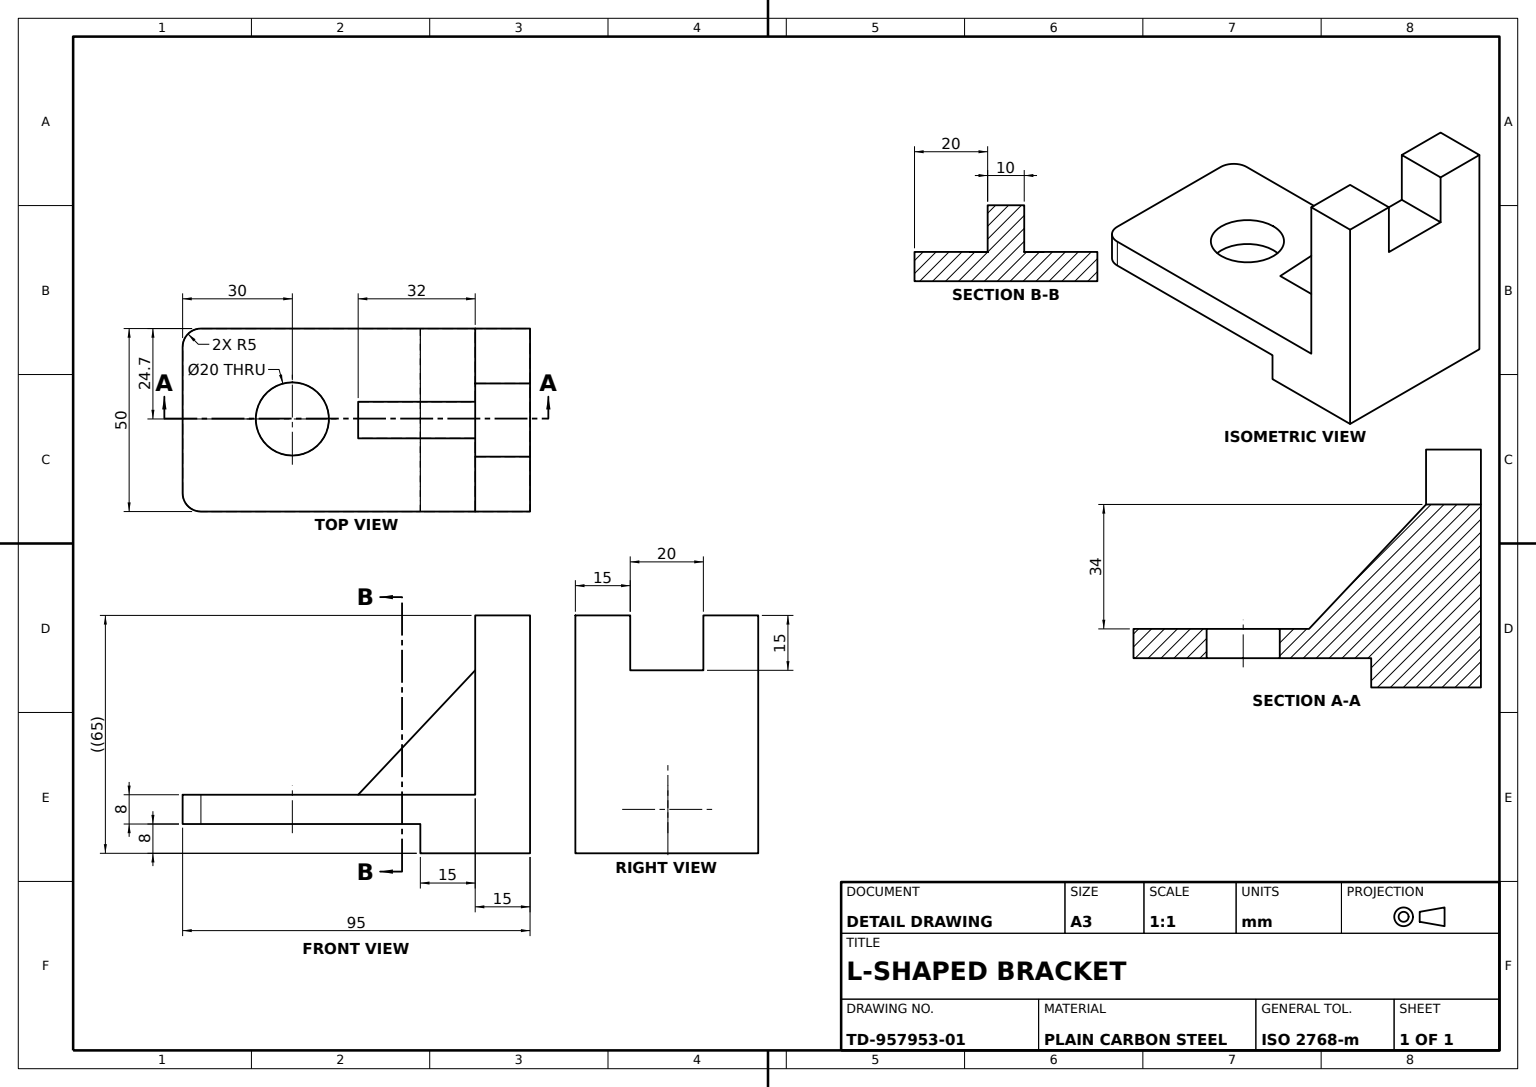
from build123d import *

# Parameters (mm, degrees)
BRACKET_BODY_DEPTH        = 50
THROUGH_HOLE_SKETCH_R     = 10
THROUGH_HOLE_DEPTH        = 50
UPRIGHT_NOTCH_20X10_DEPTH = 15
CORNER_FILLET_R5_R        = 5
SIDE_TAB_DEPTH            = 5


with BuildPart() as part:
    # Bracket L-Profile Sketch → Bracket Body (new body)
    with BuildSketch(Plane.XY):
        Polygon((0, 65), (0, 0), (-30, 0), (-30, 8), (-95, 8), (-95, 16), (-15, 16), (-15, 65), align=None)
    extrude(amount=BRACKET_BODY_DEPTH)

    # Through Hole Sketch → Through Hole (cut)
    with BuildSketch(Plane(origin=(0, 16, 0), x_dir=(1, 0, 0), z_dir=(0, 1, 0))):
        with Locations(Location((-65, -24.700639753, 0), (0, 0, 270))):
            Circle(THROUGH_HOLE_SKETCH_R)
    extrude(amount=-THROUGH_HOLE_DEPTH, mode=Mode.SUBTRACT)

    # Upright Notch Sketch → Upright Notch 20x10 (cut)
    with BuildSketch(Plane(origin=(0, 65, 0), x_dir=(1, 0, 0), z_dir=(0, 1, 0))):
        Polygon((0, -25), (0, -35), (-15, -35), (-15, -15), (0, -15), align=None)
    extrude(amount=-UPRIGHT_NOTCH_20X10_DEPTH, mode=Mode.SUBTRACT)

    # Corner Fillet R5
    corner_fillet_r5_edges = [part.edges().sort_by_distance(p)[0] for p in [
        (-95, 12, 0),
        (-95, 12, 50),
    ]]
    fillet(corner_fillet_r5_edges, radius=CORNER_FILLET_R5_R)

    # Side Tab Sketch → Side Tab (add, symmetric)
    with BuildSketch(Plane(origin=(0, 0, 25), x_dir=(-1, 0, 0), z_dir=(0, 0, -1))):
        Polygon((15, 16), (47, 16), (15, 50), align=None)
    extrude(amount=SIDE_TAB_DEPTH, both=True)


solid = part.part
